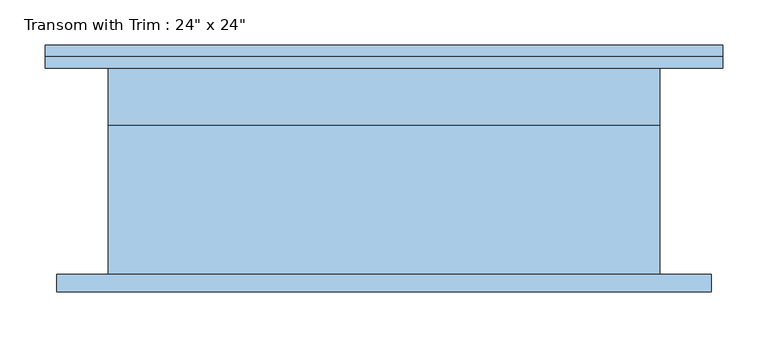
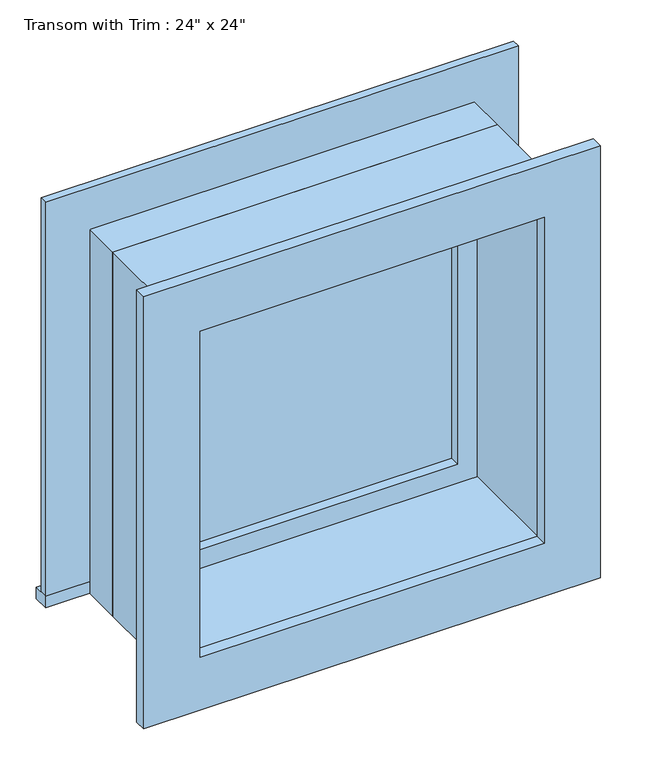
"""IFC4 building model written with IfcOpenShell, lengths in millimetres: window geometry."""

from ifc_helpers import new_model, si_unit, frame, origin, place, context, project, spatial, polyline, outline, extrude, source, transform, mapped, element, save


def window_3ed046d9(model_context):
    return source(origin(), model_context, "Body", "SweptSolid", [
        extrude(outline(polyline([(-412.75, 139.7), (336.55, 139.7), (336.55, 114.3), (-412.75, 114.3), (-412.75, 139.7)])), frame((0.0, 0.0, 2159.0), z_axis=(0.0, 0.0, 1.0), x_axis=(1.0, 0.0, 0.0)), (0.0, 0.0, 1.0), 19.05),
        extrude(outline(polyline([(2749.55, -323.85), (2749.55, 247.65), (2178.05, 247.65), (2178.05, 336.55), (2838.45, 336.55), (2838.45, -412.75), (2178.05, -412.75), (2178.05, -323.85), (2749.55, -323.85)])), frame((0.0, 114.3, 0.0), z_axis=(0.0, 1.0, 0.0), x_axis=(0.0, 0.0, 1.0)), (0.0, 0.0, 1.0), 12.7),
        extrude(outline(polyline([(2825.75, 323.85), (2825.75, -400.05), (2101.85, -400.05), (2101.85, 323.85), (2825.75, 323.85)]), holes=[polyline([(2736.85, 234.95), (2190.75, 234.95), (2190.75, -311.15), (2736.85, -311.15), (2736.85, 234.95)])]), frame((0.0, -133.35, 0.0), z_axis=(0.0, 1.0, 0.0), x_axis=(0.0, 0.0, 1.0)), (0.0, 0.0, 1.0), 19.05),
        extrude(outline(polyline([(203.2, 66.675), (-279.4, 66.675), (-279.4, 79.375), (203.2, 79.375), (203.2, 66.675)])), frame((0.0, 0.0, 2222.5), z_axis=(0.0, 0.0, 1.0), x_axis=(1.0, 0.0, 0.0)), (0.0, 0.0, 1.0), 482.6),
        extrude(outline(polyline([(2749.55, -323.85), (2178.05, -323.85), (2178.05, 247.65), (2749.55, 247.65), (2749.55, -323.85)]), holes=[polyline([(2705.1, -279.4), (2705.1, 203.2), (2222.5, 203.2), (2222.5, -279.4), (2705.1, -279.4)])]), frame((0.0, 50.8, 0.0), z_axis=(0.0, 1.0, 0.0), x_axis=(0.0, 0.0, 1.0)), (0.0, 0.0, 1.0), 44.45),
        extrude(outline(polyline([(2768.6, -342.9), (2159.0, -342.9), (2159.0, 266.7), (2768.6, 266.7), (2768.6, -342.9)]), holes=[polyline([(2736.85, -311.15), (2736.85, 234.95), (2190.75, 234.95), (2190.75, -311.15), (2736.85, -311.15)])]), frame((0.0, -114.3, 0.0), z_axis=(0.0, 1.0, 0.0), x_axis=(0.0, 0.0, 1.0)), (0.0, 0.0, 1.0), 165.1),
        extrude(outline(polyline([(2768.6, 266.7), (2768.6, -342.9), (2159.0, -342.9), (2159.0, 266.7), (2768.6, 266.7)]), holes=[polyline([(2749.55, 247.65), (2178.05, 247.65), (2178.05, -323.85), (2749.55, -323.85), (2749.55, 247.65)])]), frame((0.0, 50.8, 0.0), z_axis=(0.0, 1.0, 0.0), x_axis=(0.0, 0.0, 1.0)), (0.0, 0.0, 1.0), 63.5),
    ])


if __name__ == "__main__":
    model = new_model("IFC4")
    model_context = context("Model", 3, world=origin())
    ifc_project = project(units=[si_unit("LENGTHUNIT", "METRE", prefix="MILLI")], contexts=[model_context])
    site = spatial("IfcSite", under=ifc_project)
    building = spatial("IfcBuilding", under=site)
    placement = place(None, origin())
    window_shape = window_3ed046d9(model_context)
    element("IfcWindow", 1, ObjectType="Transom with Trim : 24\" x 24\"", at=placement, inside=building, context=model_context, shape_type="MappedRepresentation", body=[
        mapped(window_shape, transform((0.0, 0.0, 0.0), x_axis=(1.0, 0.0, 0.0), y_axis=(0.0, 1.0, 0.0), z_axis=(0.0, 0.0, 1.0))),
    ])
    save(model, "model.ifc")

# Revit data of these elements
# Type "Transom with Trim : 24\" x 24\""
#   Type Mark = "16"
#   Construction Type Id = "GSP4R"
#   Assembly Code = "B2020100"
#   Analytic Construction = "1/8 in Pilkington single glazing"
#   Visual Light Transmittance = 0.9
#   Solar Heat Gain Coefficient = 0.78
#   Heat Transfer Coefficient (U) = 0.6496 BTU/(h·ft²·°F)
#   Height = 2' - 0"
#   Default Sill Height = 7' - 1"
#   Trim Projection - Ext. = 0' - 0 1/2"
#   Trim Projection - Int. = 0' - 0 3/4"
#   Trim Width - Exterior = 0' - 3 1/2"
#   Trim Width - Interior = 0' - 3 1/2"
#   Width = 2' - 0"
#   Window Inset = 0' - 0 3/4"
#   Define Thermal Properties by = 1
#   Glass Pane Material = Glass
#   Sash Material = Sash
#   Trim Exterior Material = Trim
#   Trim Interior Material = Trim
#   Wall Closure = (empty or 0)
# Element 1 (IfcWindow, "Transom with Trim : 24\" x 24\"")
#   Materials on its faces: "Sash", "Trim", "Glass"
# Materials
#   "Glass": class "Glass", colour RGB 0 128 192, transparency 0.75, Description = "Soda Lime Glass", Cost = 0
#   "Sash": class "Wood", colour RGB 224 178 126, transparency 0
#   "Trim": class "Wood", colour RGB 224 178 126, transparency 0
